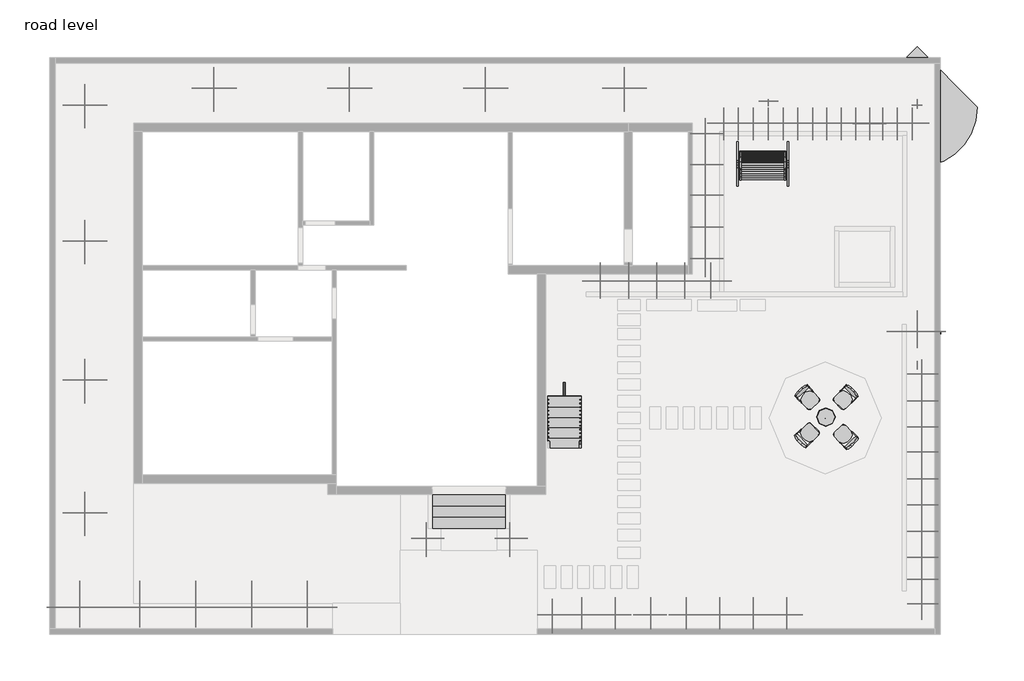
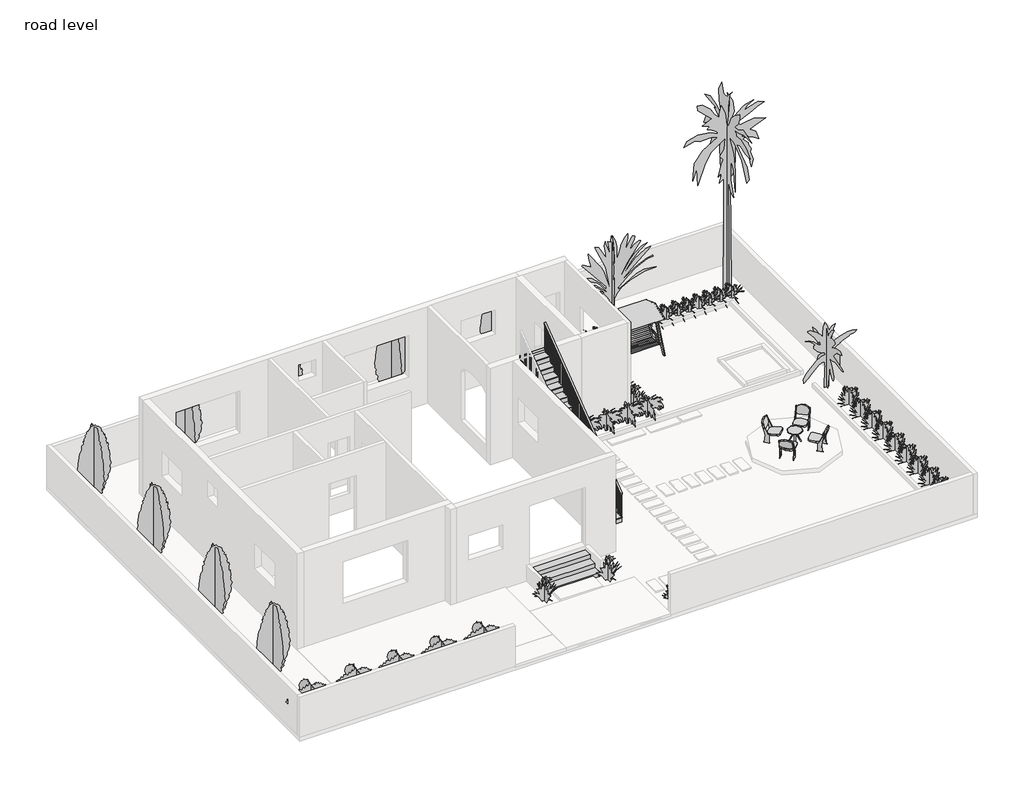
# One storey, part 3 of 3: 60 geographic elements, 7 furniture elements, 1 member, 1 railing, 1 stair flight.
# Revit data of these elements (continued)
# Type "RPC Plant - Tropical : Dagger - 2'" (continued)
#   built-in parameter 1005198 = "{2, 15},{39, RPC-16-G3A7-NEG0-UH6H-J000-ST1L-LVER-AU},{1, 0},{1, 0},{2, 35},{1, 8},{5, Color},{1, 0},{1, 0},{3, 0.8},{3, 0.8},{3, 0.8},{1, 8},{7, BBoxMin},{1, 0},{1, 0},{1, 0},{1, 0},{1, 0},{1, 8},{7, BBoxMax},{1, 0},{1, 0},{1, 0},{1, 0},{1, 0},{2, 11},{9, RPCTypeId},{1, 0},{1, 0},{39, RPC-16-G3A7-NEG0-UH6H-J000-ST1L-LVER-AU},{1, 6},{14, RPCPlantHeight},{1, 0},{1, 0},{1, 2},{2, 11},{7, keyword},{1, 0},{1, 0},{55, :Geometry:RPC:Dagger:Yucca Recurvifolia:plant:tropical.},{2, 11},{8, category},{1, 0},{1, 0},{17, :Plants [General]},{2, 11},{12, LocalizedUID},{1, 0},{1, 0},{6, Dagger},{2, 14},{6, Height},{1, 0},{1, 0},{1, 2},{1, 2},{16, Cast Reflections},{1, 0},{1, 0},{1, 0},{1, 2},{12, Cast Shadows},{1, 0},{1, 0},{1, 1},{1, 2},{9, Lock View},{1, 0},{1, 0},{1, 0},{1, 4},{5, ViewC},{1, 0},{1, 0},{1, 0},{2, 11},{20, AdvancedUIDefinition},{1, 0},{1, 0},{0, },{2, 11},{10, AssetLibID},{1, 0},{1, 0},{36, 4D3F6E72-3F99-4203-98E9-AF80B3C7A7A4},{2, 11},{10, BaseSchema},{1, 0},{1, 0},{9, RPCSchema},{2, 11},{12, ExchangeGUID},{1, 0},{1, 0},{0, },{1, 2},{6, Hidden},{1, 0},{1, 0},{1, 0},{1, 4},{11, RPCCategory},{1, 0},{1, 0},{1, 0},{2, 11},{8, RPCImage},{1, 0},{1, 0},{0, },{1, 4},{13, SchemaVersion},{1, 0},{1, 0},{1, 4},{2, 11},{12, UIDefinition},{1, 0},{1, 0},{0, },{2, 11},{6, UIName},{1, 0},{1, 0},{39, RPC-16-G3A7-NEG0-UH6H-J000-ST1L-LVER-AU},{2, 11},{11, VersionGUID},{1, 0},{1, 0},{9, RPCSchema},{2, 11},{9, assettype},{1, 0},{1, 0},{11, RPCGeometry},{2, 11},{11, description},{1, 0},{1, 0},{0, },{2, 11},{9, localname},{1, 0},{1, 0},{3, RPC},{2, 11},{9, localtype},{1, 0},{1, 0},{3, RPC},{1, 4},{8, revision},{1, 0},{1, 0},{1, 1},{2, 11},{9, thumbnail},{1, 0},{1, 0},{0, },{1, 4},{7, version},{1, 0},{1, 0},{1, 1},{1, 2},{20, RPC_Cast Reflections},{1, 0},{1, 0},{1, 1},{1, 2},{16, RPC_Cast Shadows},{1, 0},{1, 0},{1, 1},{1, 2},{13, RPC_Lock View},{1, 0},{1, 0},{1, 0},{1, 4},{9, RPC_ViewC},{1, 0},{1, 0},{1, 0},{21, assetlibrary_base.fbx},{1, 5},"
#   built-in parameter 1005195 = "RPC-16-G3A7-NEG0-UH6H-J000-ST1L-LVER-AU"
#   Type Comments = "Dagger"
#   Assembly Code = "G2050500"
#   Height = 2' - 0"
#   Default Elevation = 0
# Type "RPC Plant - Tropical : Japanese Fern - 2.5'"
#   built-in parameter 1005198 = "{2, 15},{39, RPC-16-G1GK-JAPX-7J4P-Q000-ST1L-LVER-AU},{1, 0},{1, 0},{2, 35},{1, 8},{5, Color},{1, 0},{1, 0},{3, 0.8},{3, 0.8},{3, 0.8},{1, 8},{7, BBoxMin},{1, 0},{1, 0},{1, 0},{1, 0},{1, 0},{1, 8},{7, BBoxMax},{1, 0},{1, 0},{1, 0},{1, 0},{1, 0},{2, 11},{9, RPCTypeId},{1, 0},{1, 0},{39, RPC-16-G1GK-JAPX-7J4P-Q000-ST1L-LVER-AU},{1, 6},{14, RPCPlantHeight},{1, 0},{1, 0},{3, 2.5},{2, 11},{7, keyword},{1, 0},{1, 0},{53, :Geometry:RPC:Japanese Fern:plant:small:japanese fern},{2, 11},{8, category},{1, 0},{1, 0},{17, :Shrubs [General]},{2, 11},{12, LocalizedUID},{1, 0},{1, 0},{13, Japanese Fern},{2, 14},{6, Height},{1, 0},{1, 0},{3, 2.5},{1, 2},{16, Cast Reflections},{1, 0},{1, 0},{1, 0},{1, 2},{12, Cast Shadows},{1, 0},{1, 0},{1, 1},{1, 2},{9, Lock View},{1, 0},{1, 0},{1, 0},{1, 4},{5, ViewC},{1, 0},{1, 0},{1, 0},{2, 11},{20, AdvancedUIDefinition},{1, 0},{1, 0},{0, },{2, 11},{10, AssetLibID},{1, 0},{1, 0},{36, 4D3F6E72-3F99-4203-98E9-AF80B3C7A7A4},{2, 11},{10, BaseSchema},{1, 0},{1, 0},{9, RPCSchema},{2, 11},{12, ExchangeGUID},{1, 0},{1, 0},{0, },{1, 2},{6, Hidden},{1, 0},{1, 0},{1, 0},{1, 4},{11, RPCCategory},{1, 0},{1, 0},{1, 0},{2, 11},{8, RPCImage},{1, 0},{1, 0},{0, },{1, 4},{13, SchemaVersion},{1, 0},{1, 0},{1, 4},{2, 11},{12, UIDefinition},{1, 0},{1, 0},{0, },{2, 11},{6, UIName},{1, 0},{1, 0},{39, RPC-16-G1GK-JAPX-7J4P-Q000-ST1L-LVER-AU},{2, 11},{11, VersionGUID},{1, 0},{1, 0},{9, RPCSchema},{2, 11},{9, assettype},{1, 0},{1, 0},{11, RPCGeometry},{2, 11},{11, description},{1, 0},{1, 0},{0, },{2, 11},{9, localname},{1, 0},{1, 0},{3, RPC},{2, 11},{9, localtype},{1, 0},{1, 0},{3, RPC},{1, 4},{8, revision},{1, 0},{1, 0},{1, 1},{2, 11},{9, thumbnail},{1, 0},{1, 0},{0, },{1, 4},{7, version},{1, 0},{1, 0},{1, 1},{1, 2},{20, RPC_Cast Reflections},{1, 0},{1, 0},{1, 1},{1, 2},{16, RPC_Cast Shadows},{1, 0},{1, 0},{1, 1},{1, 2},{13, RPC_Lock View},{1, 0},{1, 0},{1, 0},{1, 4},{9, RPC_ViewC},{1, 0},{1, 0},{1, 0},{21, assetlibrary_base.fbx},{1, 5},"
#   built-in parameter 1005195 = "RPC-16-G1GK-JAPX-7J4P-Q000-ST1L-LVER-AU"
#   Type Comments = "Japanese Fern"
#   Assembly Code = "G2050500"
#   Height = 2' - 6"
#   Default Elevation = 0
# Type "RPC Plant - Tropical : Jungle Flame - 3'"
#   built-in parameter 1005198 = "{2, 15},{39, RPC-16-FUVJ-JWG0-MWGK-8000-ST1L-LVER-AU},{1, 0},{1, 0},{2, 35},{1, 8},{5, Color},{1, 0},{1, 0},{3, 0.8},{3, 0.8},{3, 0.8},{1, 8},{7, BBoxMin},{1, 0},{1, 0},{1, 0},{1, 0},{1, 0},{1, 8},{7, BBoxMax},{1, 0},{1, 0},{1, 0},{1, 0},{1, 0},{2, 11},{9, RPCTypeId},{1, 0},{1, 0},{39, RPC-16-FUVJ-JWG0-MWGK-8000-ST1L-LVER-AU},{1, 6},{14, RPCPlantHeight},{1, 0},{1, 0},{1, 3},{2, 11},{7, keyword},{1, 0},{1, 0},{90, :Geometry:RPC:Jungle Flame:ixora macrothyrsa:jungle flame:bush:shrub:plant:flower:tropical},{2, 11},{8, category},{1, 0},{1, 0},{17, :Shrubs [General]},{2, 11},{12, LocalizedUID},{1, 0},{1, 0},{12, Jungle Flame},{2, 14},{6, Height},{1, 0},{1, 0},{1, 3},{1, 2},{16, Cast Reflections},{1, 0},{1, 0},{1, 0},{1, 2},{12, Cast Shadows},{1, 0},{1, 0},{1, 1},{1, 2},{9, Lock View},{1, 0},{1, 0},{1, 0},{1, 4},{5, ViewC},{1, 0},{1, 0},{1, 0},{2, 11},{20, AdvancedUIDefinition},{1, 0},{1, 0},{0, },{2, 11},{10, AssetLibID},{1, 0},{1, 0},{36, 4D3F6E72-3F99-4203-98E9-AF80B3C7A7A4},{2, 11},{10, BaseSchema},{1, 0},{1, 0},{9, RPCSchema},{2, 11},{12, ExchangeGUID},{1, 0},{1, 0},{0, },{1, 2},{6, Hidden},{1, 0},{1, 0},{1, 0},{1, 4},{11, RPCCategory},{1, 0},{1, 0},{1, 0},{2, 11},{8, RPCImage},{1, 0},{1, 0},{0, },{1, 4},{13, SchemaVersion},{1, 0},{1, 0},{1, 4},{2, 11},{12, UIDefinition},{1, 0},{1, 0},{0, },{2, 11},{6, UIName},{1, 0},{1, 0},{39, RPC-16-FUVJ-JWG0-MWGK-8000-ST1L-LVER-AU},{2, 11},{11, VersionGUID},{1, 0},{1, 0},{9, RPCSchema},{2, 11},{9, assettype},{1, 0},{1, 0},{11, RPCGeometry},{2, 11},{11, description},{1, 0},{1, 0},{0, },{2, 11},{9, localname},{1, 0},{1, 0},{3, RPC},{2, 11},{9, localtype},{1, 0},{1, 0},{3, RPC},{1, 4},{8, revision},{1, 0},{1, 0},{1, 1},{2, 11},{9, thumbnail},{1, 0},{1, 0},{0, },{1, 4},{7, version},{1, 0},{1, 0},{1, 1},{1, 2},{20, RPC_Cast Reflections},{1, 0},{1, 0},{1, 1},{1, 2},{16, RPC_Cast Shadows},{1, 0},{1, 0},{1, 1},{1, 2},{13, RPC_Lock View},{1, 0},{1, 0},{1, 0},{1, 4},{9, RPC_ViewC},{1, 0},{1, 0},{1, 0},{21, assetlibrary_base.fbx},{1, 5},"
#   built-in parameter 1005195 = "RPC-16-FUVJ-JWG0-MWGK-8000-ST1L-LVER-AU"
#   Type Comments = "Jungle Flame"
#   Assembly Code = "G2050500"
#   Height = 3' - 0"
#   Default Elevation = 0
# Type "RPC Tree - Deciduous : Japanese Cherry - 15'"
#   built-in parameter 1005195 = "RPC-16-FUM3-UUQ0-UBF0-N000-ST1L-LVER-AU"
#   Type Comments = "Japanese Cherry"
#   Assembly Code = "G2050500"
#   Height = 9' - 0"
#   Default Elevation = 0
# Type "RPC Tree - Tropical : Cuban Royal Palm - 25'"
#   built-in parameter 1005198 = "{2, 15},{39, RPC-16-FVGV-NKG0-7NHH-C000-ST1L-LVER-AU},{1, 0},{1, 0},{2, 35},{1, 8},{5, Color},{1, 0},{1, 0},{3, 0.8},{3, 0.8},{3, 0.8},{1, 8},{7, BBoxMin},{1, 0},{1, 0},{1, 0},{1, 0},{1, 0},{1, 8},{7, BBoxMax},{1, 0},{1, 0},{1, 0},{1, 0},{1, 0},{2, 11},{9, RPCTypeId},{1, 0},{1, 0},{39, RPC-16-FVGV-NKG0-7NHH-C000-ST1L-LVER-AU},{1, 6},{14, RPCPlantHeight},{1, 0},{1, 0},{2, 25},{2, 11},{7, keyword},{1, 0},{1, 0},{72, :Geometry:RPC:Cuban Royal Palm:Roystonea regia (Oreodoxa):palm:tropical.},{2, 11},{8, category},{1, 0},{1, 0},{17, :Trees [Tropical]},{2, 11},{12, LocalizedUID},{1, 0},{1, 0},{16, Cuban Royal Palm},{2, 14},{6, Height},{1, 0},{1, 0},{2, 25},{1, 2},{16, Cast Reflections},{1, 0},{1, 0},{1, 0},{1, 2},{12, Cast Shadows},{1, 0},{1, 0},{1, 1},{1, 2},{9, Lock View},{1, 0},{1, 0},{1, 0},{1, 4},{5, ViewC},{1, 0},{1, 0},{1, 0},{2, 11},{20, AdvancedUIDefinition},{1, 0},{1, 0},{0, },{2, 11},{10, AssetLibID},{1, 0},{1, 0},{36, 4D3F6E72-3F99-4203-98E9-AF80B3C7A7A4},{2, 11},{10, BaseSchema},{1, 0},{1, 0},{9, RPCSchema},{2, 11},{12, ExchangeGUID},{1, 0},{1, 0},{0, },{1, 2},{6, Hidden},{1, 0},{1, 0},{1, 0},{1, 4},{11, RPCCategory},{1, 0},{1, 0},{1, 0},{2, 11},{8, RPCImage},{1, 0},{1, 0},{0, },{1, 4},{13, SchemaVersion},{1, 0},{1, 0},{1, 4},{2, 11},{12, UIDefinition},{1, 0},{1, 0},{0, },{2, 11},{6, UIName},{1, 0},{1, 0},{39, RPC-16-FVGV-NKG0-7NHH-C000-ST1L-LVER-AU},{2, 11},{11, VersionGUID},{1, 0},{1, 0},{9, RPCSchema},{2, 11},{9, assettype},{1, 0},{1, 0},{11, RPCGeometry},{2, 11},{11, description},{1, 0},{1, 0},{0, },{2, 11},{9, localname},{1, 0},{1, 0},{3, RPC},{2, 11},{9, localtype},{1, 0},{1, 0},{3, RPC},{1, 4},{8, revision},{1, 0},{1, 0},{1, 1},{2, 11},{9, thumbnail},{1, 0},{1, 0},{0, },{1, 4},{7, version},{1, 0},{1, 0},{1, 1},{1, 2},{20, RPC_Cast Reflections},{1, 0},{1, 0},{1, 1},{1, 2},{16, RPC_Cast Shadows},{1, 0},{1, 0},{1, 1},{1, 2},{13, RPC_Lock View},{1, 0},{1, 0},{1, 0},{1, 4},{9, RPC_ViewC},{1, 0},{1, 0},{1, 0},{21, assetlibrary_base.fbx},{1, 5},"
#   built-in parameter 1005195 = "RPC-16-FVGV-NKG0-7NHH-C000-ST1L-LVER-AU"
#   Type Comments = "Cuban Royal Palm"
#   Assembly Code = "G2050500"
#   Height = 25' - 0"
#   Plan Symbol = element 455244
#   Default Elevation = 0
# Type "RPC Tree - Tropical : Japanese Fiber Banana - 8'"
#   built-in parameter 1005198 = "{2, 15},{39, RPC-16-FVGT-NR7X-7G1M-A000-ST1L-LVER-AU},{1, 0},{1, 0},{2, 35},{1, 8},{5, Color},{1, 0},{1, 0},{3, 0.8},{3, 0.8},{3, 0.8},{1, 8},{7, BBoxMin},{1, 0},{1, 0},{1, 0},{1, 0},{1, 0},{1, 8},{7, BBoxMax},{1, 0},{1, 0},{1, 0},{1, 0},{1, 0},{2, 11},{9, RPCTypeId},{1, 0},{1, 0},{39, RPC-16-FVGT-NR7X-7G1M-A000-ST1L-LVER-AU},{1, 6},{14, RPCPlantHeight},{1, 0},{1, 0},{1, 8},{2, 11},{7, keyword},{1, 0},{1, 0},{62, :Geometry:RPC:Japanese Fiber Banana:Musa basjoo:Tree:Tropical.},{2, 11},{8, category},{1, 0},{1, 0},{17, :Trees [Tropical]},{2, 11},{12, LocalizedUID},{1, 0},{1, 0},{21, Japanese Fiber Banana},{2, 14},{6, Height},{1, 0},{1, 0},{1, 8},{1, 2},{16, Cast Reflections},{1, 0},{1, 0},{1, 0},{1, 2},{12, Cast Shadows},{1, 0},{1, 0},{1, 1},{1, 2},{9, Lock View},{1, 0},{1, 0},{1, 0},{1, 4},{5, ViewC},{1, 0},{1, 0},{1, 0},{2, 11},{20, AdvancedUIDefinition},{1, 0},{1, 0},{0, },{2, 11},{10, AssetLibID},{1, 0},{1, 0},{36, 4D3F6E72-3F99-4203-98E9-AF80B3C7A7A4},{2, 11},{10, BaseSchema},{1, 0},{1, 0},{9, RPCSchema},{2, 11},{12, ExchangeGUID},{1, 0},{1, 0},{0, },{1, 2},{6, Hidden},{1, 0},{1, 0},{1, 0},{1, 4},{11, RPCCategory},{1, 0},{1, 0},{1, 0},{2, 11},{8, RPCImage},{1, 0},{1, 0},{0, },{1, 4},{13, SchemaVersion},{1, 0},{1, 0},{1, 4},{2, 11},{12, UIDefinition},{1, 0},{1, 0},{0, },{2, 11},{6, UIName},{1, 0},{1, 0},{39, RPC-16-FVGT-NR7X-7G1M-A000-ST1L-LVER-AU},{2, 11},{11, VersionGUID},{1, 0},{1, 0},{9, RPCSchema},{2, 11},{9, assettype},{1, 0},{1, 0},{11, RPCGeometry},{2, 11},{11, description},{1, 0},{1, 0},{0, },{2, 11},{9, localname},{1, 0},{1, 0},{3, RPC},{2, 11},{9, localtype},{1, 0},{1, 0},{3, RPC},{1, 4},{8, revision},{1, 0},{1, 0},{1, 1},{2, 11},{9, thumbnail},{1, 0},{1, 0},{0, },{1, 4},{7, version},{1, 0},{1, 0},{1, 1},{1, 2},{20, RPC_Cast Reflections},{1, 0},{1, 0},{1, 1},{1, 2},{16, RPC_Cast Shadows},{1, 0},{1, 0},{1, 1},{1, 2},{13, RPC_Lock View},{1, 0},{1, 0},{1, 0},{1, 4},{9, RPC_ViewC},{1, 0},{1, 0},{1, 0},{21, assetlibrary_base.fbx},{1, 5},"
#   built-in parameter 1005195 = "RPC-16-FVGT-NR7X-7G1M-A000-ST1L-LVER-AU"
#   Type Comments = "Japanese Fiber Banana"
#   Assembly Code = "G2050500"
#   Height = 8' - 0"
#   Plan Symbol = element 455244
#   Default Elevation = 0
# Type "RPC Tree - Tropical : Orange Tree - 11'"
#   built-in parameter 1005195 = "RPC-16-G2M6-EAFX-C5H6-W000-ST1L-LVER-AU"
#   Type Comments = "Orange Tree"
#   Assembly Code = "G2050500"
#   Height = 11' - 0"
#   Plan Symbol = element 455245
#   Default Elevation = 0
# Type "Handrail - Rectangular"
#   Assembly Code = "C2010400"
#   built-in parameter 1008612 = 0.0416667 (stored number, unit not read)
#   built-in parameter 1008611 = 0.0416667 (stored number, unit not read)
#   built-in parameter 1008609 = 0.333333 (stored number, unit not read)
#   built-in parameter 1008604 = 0.166667 (stored number, unit not read)
#   built-in parameter 1008603 = 0.166667 (stored number, unit not read)
#   Railing Height = 3' - 0"
#   built-in parameter 1008630 = 2
#   built-in parameter 1008610 = 2
#   built-in parameter 1008618 = Baluster - Square : 3/4"
# Element 1 (IfcFurniture, "0610 x 0160mm")
#   Phase Created = New Construction
#   Materials on its faces: "wood finish", "steel", "Laminate - Ivory, Matte", "fabric"
# Element 2 (IfcFurniture, "Casework 1 : Casework 1")
#   Phase Created = New Construction
#   Materials on its faces: "Concrete, Cast-in-Place gray"
# Elements 3, 4, 5, 6 (IfcFurniture, "Seating-Auditorium : 18\" x 24\" x 30\"")
#   Phase Created = New Construction
#   Materials on its faces: "Steel, Paint Finish, Dark Gray, Matte", "Linen, Beige"
# Element 7 (IfcFurniture, "Table-Trio End : 20\" Diameter")
#   Phase Created = New Construction
#   Materials on its faces: "Wood - Birch", "Laminate - Ivory,Matte"
# Elements 8, 9, 10, 11, 12, 13, 14, 15, 16, 17, 18, 19, 20 (IfcGeographicElement, "RPC Plant - Tropical")
#   Phase Created = New Construction
# Elements 21, 22, 23, 24, 25, 26, 27, 28, 29, 30, 31, 32, 33, 34 (IfcGeographicElement, "RPC Plant - Tropical : Agave - 1.5'")
#   Phase Created = New Construction
# Elements 35, 36, 37, 38, 39, 40, 41, 42, 43, 44 (IfcGeographicElement, "RPC Plant - Tropical : Dagger - 2'")
#   Phase Created = New Construction
# Elements 45, 46, 47, 48, 49 (IfcGeographicElement, "RPC Plant - Tropical : Japanese Fern - 2.5'")
#   Phase Created = New Construction
# Elements 50, 51, 52, 53, 54, 55, 56 (IfcGeographicElement, "RPC Plant - Tropical : Jungle Flame - 3'")
#   Phase Created = New Construction
# Elements 57, 58, 59, 60, 61, 62, 63, 64 (IfcGeographicElement, "RPC Tree - Deciduous : Japanese Cherry - 15'")
#   Phase Created = New Construction
# Element 65 (IfcGeographicElement, "RPC Tree - Tropical : Cuban Royal Palm - 25'")
#   Phase Created = New Construction
# Element 66 (IfcGeographicElement, "RPC Tree - Tropical : Japanese Fiber Banana - 8'")
#   Phase Created = New Construction
# Element 67 (IfcGeographicElement, "RPC Tree - Tropical : Orange Tree - 11'")
#   Phase Created = New Construction
# Element 68 (IfcMember, "Carriage - 2\" Width")
#   Phase Created = New Construction
# Element 69 (IfcRailing, "Handrail - Rectangular")
#   Phase Created = New Construction
# Element 70 (IfcStairFlight, "2\" Tread 1\" Nosing 1/4\" Riser")
#   Phase Created = New Construction
# Materials
#   "Wood - Birch": colour RGB 230 196 162, transparency 0
#   "Laminate - Ivory, Matte": colour RGB 247 247 239, transparency 0
#   "Linen, Beige": class "Textile", colour RGB 249 239 230, transparency 0, Description = "Linen, beige", Cost = 0
#   "Steel, Paint Finish, Dark Gray, Matte": class "Metal", colour RGB 0 0 0, transparency 0, Description = "Steel, paint finish, dark gray, matte", Cost = 0
#   "Laminate - Ivory,Matte": colour RGB 247 247 239, transparency 0
#   "wood finish": class "Generic", colour RGB 120 120 120, transparency 0, Cost = 0
#   "steel": class "Generic", colour RGB 120 120 120, transparency 0, Cost = 0
#   "fabric": class "Generic", colour RGB 120 120 120, transparency 0, Cost = 0
#   "Concrete, Cast-in-Place gray": class "Concrete", colour RGB 192 192 192, transparency 0, Description = "Cast-in-place concrete", Cost = 0
